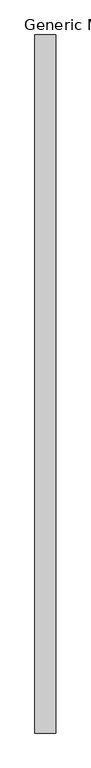
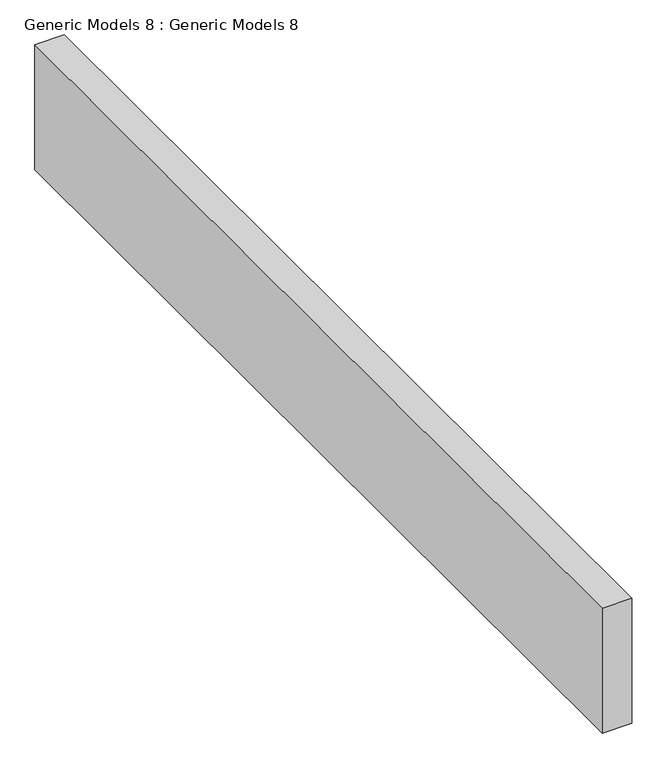
"""IFC4 building model written with IfcOpenShell, lengths in millimetres: proxy geometry, Generic Models 8 : Generic Models 8."""

from ifc_helpers import new_model, si_unit, frame, origin, place, context, project, spatial, polyline, outline, extrude, source, transform, mapped, element, save


def generic_models_8_generic_models_8_1b8929a2(model_context):
    return source(origin(), model_context, "Body", "SweptSolid", [
        extrude(outline(polyline([(1022.326752, 139.1133697), (1022.326752, -4077.2866303), (895.326752, -4077.2866303), (895.326752, 139.1133697), (1022.326752, 139.1133697)])), frame((0.0, 0.0, 2996.4723824), z_axis=(0.0, 0.0, 1.0), x_axis=(1.0, 0.0, 0.0)), (0.0, 0.0, 1.0), 566.7847605),
    ])


if __name__ == "__main__":
    model = new_model("IFC4")
    model_context = context("Model", 3, world=origin())
    ifc_project = project(units=[si_unit("LENGTHUNIT", "METRE", prefix="MILLI")], contexts=[model_context])
    site = spatial("IfcSite", under=ifc_project)
    building = spatial("IfcBuilding", under=site)
    placement = place(None, origin())
    generic_models_8_generic_models_8_shape = generic_models_8_generic_models_8_1b8929a2(model_context)
    element("IfcBuildingElementProxy", 1, Name="Generic Models 8 : Generic Models 8", ObjectType="Generic Models 8 : Generic Models 8", at=placement, inside=building, context=model_context, shape_type="MappedRepresentation", body=[
        mapped(generic_models_8_generic_models_8_shape, transform((0.0, 0.0, 0.0), x_axis=(1.0, 0.0, 0.0), y_axis=(0.0, 1.0, 0.0), z_axis=(0.0, 0.0, 1.0))),
    ])
    save(model, "model.ifc")

# Revit data of these elements
# Element 1 (IfcBuildingElementProxy, "Generic Models 8 : Generic Models 8")
#   Materials on its faces: "Clad - White"
# Materials
#   "Clad - White": class "Wood", colour RGB 242 242 238, transparency 0, Cost = 0
